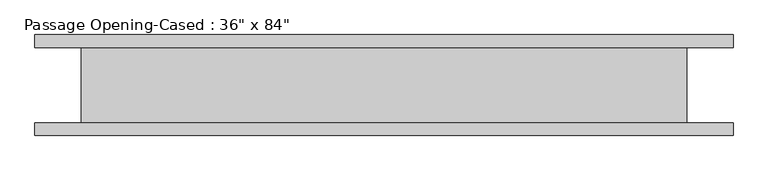
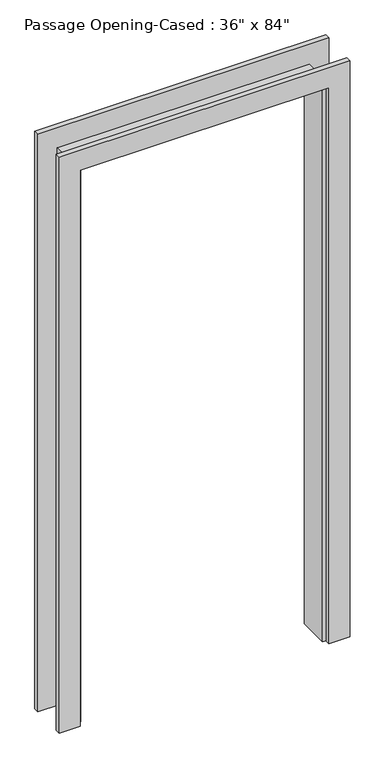
"""IFC4 building model written with IfcOpenShell, lengths in millimetres: proxy geometry."""

from ifc_helpers import new_model, si_unit, frame, origin, place, context, project, spatial, polyline, outline, extrude, faceted_brep, source, transform, mapped, element, save


def proxy_99694262(model_context):
    return source(origin(), model_context, "Body", "SolidModel", [
        faceted_brep([(429.9613433, 57.15, 0.0), (449.0113433, 57.15, 0.0), (449.0113433, -57.15, 0.0), (429.9613433, -57.15, 0.0), (429.9613433, 57.15, 2114.55), (449.0113433, 57.15, 2133.6), (449.0113433, -57.15, 2133.6), (429.9613433, -57.15, 2114.55), (-446.3386567, 57.15, 2114.55), (-465.3886567, 57.15, 2133.6), (-465.3886567, -57.15, 2133.6), (-446.3386567, -57.15, 2114.55), (-446.3386567, 57.15, 0.0), (-446.3386567, -57.15, 0.0), (-465.3886567, -57.15, 0.0), (-465.3886567, 57.15, 0.0)], [[[0, 1, 2, 3]], [[1, 0, 4, 5]], [[2, 1, 5, 6]], [[3, 2, 6, 7]], [[0, 3, 7, 4]], [[5, 4, 8, 9]], [[6, 5, 9, 10]], [[7, 6, 10, 11]], [[4, 7, 11, 8]], [[12, 13, 14, 15]], [[9, 8, 12, 15]], [[10, 9, 15, 14]], [[11, 10, 14, 13]], [[8, 11, 13, 12]]]),
        extrude(outline(polyline([(0.0, 518.8613433), (2209.8, 518.8613433), (2209.8, -535.2386567), (0.0, -535.2386567), (0.0, -459.0386567), (2127.25, -459.0386567), (2127.25, 442.6613433), (0.0, 442.6613433), (0.0, 518.8613433)])), frame((0.0, 57.15, 0.0), z_axis=(0.0, 1.0, 0.0), x_axis=(0.0, 0.0, 1.0)), (0.0, 0.0, 1.0), 19.05),
        extrude(outline(polyline([(0.0, -459.0386567), (2127.25, -459.0386567), (2127.25, 442.6613433), (0.0, 442.6613433), (0.0, 518.8613433), (2203.45, 518.8613433), (2203.45, -535.2386567), (0.0, -535.2386567), (0.0, -459.0386567)])), frame((0.0, -76.2, 0.0), z_axis=(0.0, 1.0, 0.0), x_axis=(0.0, 0.0, 1.0)), (0.0, 0.0, 1.0), 19.05),
    ])


if __name__ == "__main__":
    model = new_model("IFC4")
    model_context = context("Model", 3, world=origin())
    ifc_project = project(units=[si_unit("LENGTHUNIT", "METRE", prefix="MILLI")], contexts=[model_context])
    site = spatial("IfcSite", under=ifc_project)
    building = spatial("IfcBuilding", under=site)
    placement = place(None, origin())
    proxy_shape = proxy_99694262(model_context)
    element("IfcBuildingElementProxy", 1, Name="Passage Opening-Cased : 36\" x 84\"", ObjectType="Passage Opening-Cased : 36\" x 84\"", at=placement, inside=building, context=model_context, shape_type="MappedRepresentation", body=[
        mapped(proxy_shape, transform((0.0, 0.0, 0.0), x_axis=(1.0, 0.0, 0.0), y_axis=(0.0, 1.0, 0.0), z_axis=(0.0, 0.0, 1.0))),
    ])
    save(model, "model.ifc")

# Revit data of these elements
# Type "Passage Opening-Cased : 36\" x 84\""
#   Height = 7' - 0"
#   Trim Thickness = 0' - 0 3/4"
#   Trim Width = 0' - 3"
#   Width = 3' - 0"
#   Frame Material = Door - Frame
#   Default Elevation = 0
# Element 1 (IfcBuildingElementProxy, "Passage Opening-Cased : 36\" x 84\"")
#   Materials on its faces: "Door - Frame"
# Materials
#   "Door - Frame": colour RGB 118 70 51, transparency 0, Cost = 0
